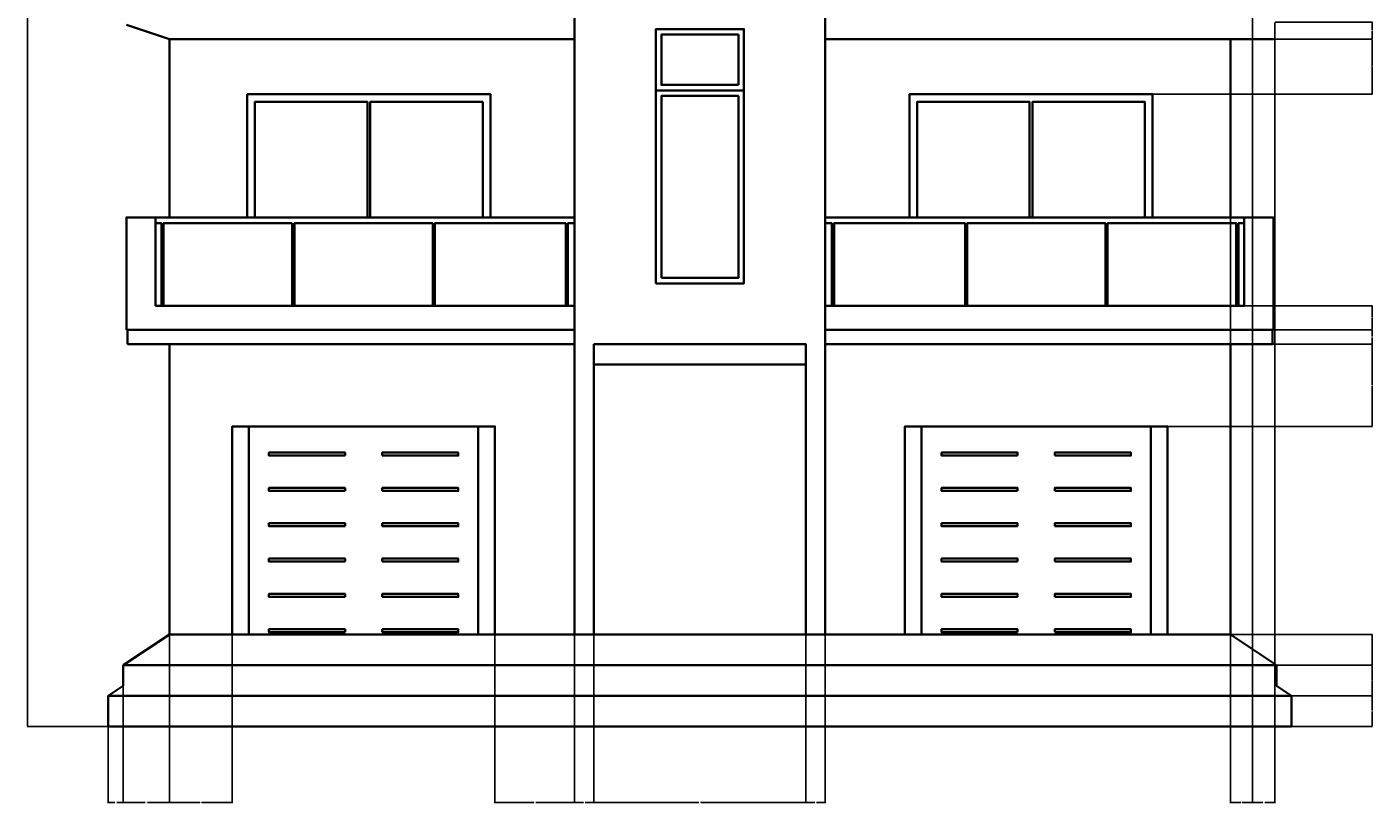
# Model space of a CAD drawing. Units: feet. Extents: x 2893 to 4112, y 897 to 1573.
# Tile 6 of 7: x 3556 to 4112, y 897 to 1218. Entities that reach past the tile are written whole.
import ezdxf

# ---------------------------------------------------------------- set-up
doc = ezdxf.new("R2010")
doc.units = ezdxf.units.FT
doc.layers.add('A-ANNO-DIMS', color=2, linetype='Continuous', lineweight=18)
doc.layers.add('A-ELEV', color=7, linetype='Continuous', lineweight=35)
doc.styles.get("Standard").update_dxf_attribs({"font": 'arial.ttf'})
doc.dimstyles.get("Standard").update_dxf_attribs({"dimtxt": 0.18, "dimasz": 0.18, "dimexe": 0.18, "dimexo": 0.0625, "dimgap": 0.09, "dimtad": 0, "dimtih": 1, "dimtoh": 1, "dimdec": 1, "dimzin": 0, "dimdsep": 46, "dimlunit": 3, "dimtxsty": 'Standard', "dimcen": 0.09, "dimadec": 0, "dimazin": 0, "dimtfac": 1, "dimtdec": 1, "dimtofl": 0, "dimtmove": 0, "dimatfit": 3, "dimfxl": 1, "dimtolj": 1, "dimtzin": 0, "dimarcsym": 0})

# ---------------------------------------------------------------- blocks, each defined once
blk = doc.blocks.new('*D14')
at = {"layer": 'A-ANNO-DIMS', "color": 0, "lineweight": -2, "transparency": 16777216}
for p, q in [((3587.66, 1527.89), (3556.04, 1527.89)), ((3556.22, 1527.71), (3556.22, 1228.65)), ((3556.22, 929.23), (3556.22, 1228.29)), ((3589.45, 929.05), (3556.04, 929.05))]:
    blk.add_line(p, q, dxfattribs=at)
at = {"layer": 'A-ANNO-DIMS', "color": 0, "transparency": 16777216}
for points in [[(3556.19, 1527.71), (3556.25, 1527.71), (3556.22, 1527.89)], [(3556.19, 929.23), (3556.25, 929.23), (3556.22, 929.05)]]:
    blk.add_solid(points, dxfattribs=at)
at = {"layer": 'Defpoints', "color": 0, "transparency": 16777216}
for p in [(3556.22, 1527.89), (3587.72, 1527.89), (3589.51, 929.05)]:
    blk.add_point(p, dxfattribs=at)
at = {"layer": 'A-ANNO-DIMS', "color": 0, "transparency": 16777216, "insert": (3556.22, 1228.47), "char_height": 0.18, "attachment_point": 5}
blk.add_mtext('\\A1;598.8', dxfattribs=at)
blk = doc.blocks.new('*D16')
at = {"layer": 'A-ANNO-DIMS', "color": 0, "lineweight": -2, "transparency": 16777216}
for p, q in [((3595.77, 954.3), (3595.77, 897.37)), ((3589.51, 941.64), (3589.51, 897.37)), ((3589.69, 897.55), (3592.25, 897.55)), ((3595.59, 897.55), (3593.03, 897.55))]:
    blk.add_line(p, q, dxfattribs=at)
at = {"layer": 'A-ANNO-DIMS', "color": 0, "transparency": 16777216}
for points in [[(3589.69, 897.58), (3589.69, 897.52), (3589.51, 897.55)], [(3595.59, 897.58), (3595.59, 897.52), (3595.77, 897.55)]]:
    blk.add_solid(points, dxfattribs=at)
at = {"layer": 'Defpoints', "color": 0, "transparency": 16777216}
for p in [(3595.77, 954.36), (3589.51, 941.7), (3595.77, 897.55)]:
    blk.add_point(p, dxfattribs=at)
at = {"layer": 'A-ANNO-DIMS', "color": 0, "transparency": 16777216, "insert": (3592.64, 897.55), "char_height": 0.18, "attachment_point": 5}
blk.add_mtext('\\A1;6.263', dxfattribs=at)
blk = doc.blocks.new('*D17')
at = {"layer": 'A-ANNO-DIMS', "color": 0, "lineweight": -2, "transparency": 16777216}
for p, q in [((3614.84, 966.95), (3614.84, 897.37)), ((3595.77, 954.3), (3595.77, 897.37)), ((3595.95, 897.55), (3604.85, 897.55)), ((3614.66, 897.55), (3605.76, 897.55))]:
    blk.add_line(p, q, dxfattribs=at)
at = {"layer": 'A-ANNO-DIMS', "color": 0, "transparency": 16777216}
for points in [[(3595.95, 897.58), (3595.95, 897.52), (3595.77, 897.55)], [(3614.66, 897.58), (3614.66, 897.52), (3614.84, 897.55)]]:
    blk.add_solid(points, dxfattribs=at)
at = {"layer": 'Defpoints', "color": 0, "transparency": 16777216}
for p in [(3614.84, 967.01), (3595.77, 954.36), (3614.84, 897.55)]:
    blk.add_point(p, dxfattribs=at)
at = {"layer": 'A-ANNO-DIMS', "color": 0, "transparency": 16777216, "insert": (3605.3, 897.55), "char_height": 0.18, "attachment_point": 5}
blk.add_mtext('\\A1;19.063', dxfattribs=at)
blk = doc.blocks.new('*D18')
at = {"layer": 'A-ANNO-DIMS', "color": 0, "lineweight": -2, "transparency": 16777216}
for p, q in [((3614.84, 966.95), (3614.84, 897.37)), ((3640.81, 966.95), (3640.81, 897.37)), ((3615.02, 897.55), (3627.43, 897.55)), ((3640.63, 897.55), (3628.22, 897.55))]:
    blk.add_line(p, q, dxfattribs=at)
at = {"layer": 'A-ANNO-DIMS', "color": 0, "transparency": 16777216}
for points in [[(3615.02, 897.58), (3615.02, 897.52), (3614.84, 897.55)], [(3640.63, 897.58), (3640.63, 897.52), (3640.81, 897.55)]]:
    blk.add_solid(points, dxfattribs=at)
at = {"layer": 'Defpoints', "color": 0, "transparency": 16777216}
for p in [(3614.84, 967.01), (3640.81, 967.01), (3640.81, 897.55)]:
    blk.add_point(p, dxfattribs=at)
at = {"layer": 'A-ANNO-DIMS', "color": 0, "transparency": 16777216, "insert": (3627.82, 897.55), "char_height": 0.18, "attachment_point": 5}
blk.add_mtext('\\A1;25.98', dxfattribs=at)
blk = doc.blocks.new('*D19')
at = {"layer": 'A-ANNO-DIMS', "color": 0, "lineweight": -2, "transparency": 16777216}
for p, q in [((3749.39, 966.95), (3749.39, 897.37)), ((3782.33, 966.95), (3782.33, 897.37)), ((3749.57, 897.55), (3765.47, 897.55)), ((3782.15, 897.55), (3766.25, 897.55))]:
    blk.add_line(p, q, dxfattribs=at)
at = {"layer": 'A-ANNO-DIMS', "color": 0, "transparency": 16777216}
for points in [[(3749.57, 897.58), (3749.57, 897.52), (3749.39, 897.55)], [(3782.15, 897.58), (3782.15, 897.52), (3782.33, 897.55)]]:
    blk.add_solid(points, dxfattribs=at)
at = {"layer": 'Defpoints', "color": 0, "transparency": 16777216}
for p in [(3749.39, 967.01), (3782.33, 967.01), (3782.33, 897.55)]:
    blk.add_point(p, dxfattribs=at)
at = {"layer": 'A-ANNO-DIMS', "color": 0, "transparency": 16777216, "insert": (3765.86, 897.55), "char_height": 0.18, "attachment_point": 5}
blk.add_mtext('\\A1;32.94', dxfattribs=at)
blk = doc.blocks.new('*D20')
at = {"layer": 'A-ANNO-DIMS', "color": 0, "lineweight": -2, "transparency": 16777216}
for p, q in [((3782.33, 966.95), (3782.33, 897.37)), ((3790.32, 966.95), (3790.32, 897.37)), ((3782.51, 897.55), (3786, 897.55)), ((3790.14, 897.55), (3786.65, 897.55))]:
    blk.add_line(p, q, dxfattribs=at)
at = {"layer": 'A-ANNO-DIMS', "color": 0, "transparency": 16777216}
for points in [[(3782.51, 897.58), (3782.51, 897.52), (3782.33, 897.55)], [(3790.14, 897.58), (3790.14, 897.52), (3790.32, 897.55)]]:
    blk.add_solid(points, dxfattribs=at)
at = {"layer": 'Defpoints', "color": 0, "transparency": 16777216}
for p in [(3782.33, 967.01), (3790.32, 967.01), (3790.32, 897.55)]:
    blk.add_point(p, dxfattribs=at)
at = {"layer": 'A-ANNO-DIMS', "color": 0, "transparency": 16777216, "insert": (3786.32, 897.55), "char_height": 0.18, "attachment_point": 5}
blk.add_mtext('\\A1;7.99', dxfattribs=at)
blk = doc.blocks.new('*D21')
at = {"layer": 'A-ANNO-DIMS', "color": 0, "lineweight": -2, "transparency": 16777216}
for p, q in [((3790.32, 966.95), (3790.32, 897.37)), ((3877.97, 966.95), (3877.97, 897.37)), ((3790.5, 897.55), (3833.75, 897.55)), ((3877.79, 897.55), (3834.54, 897.55))]:
    blk.add_line(p, q, dxfattribs=at)
at = {"layer": 'A-ANNO-DIMS', "color": 0, "transparency": 16777216}
for points in [[(3790.5, 897.58), (3790.5, 897.52), (3790.32, 897.55)], [(3877.79, 897.58), (3877.79, 897.52), (3877.97, 897.55)]]:
    blk.add_solid(points, dxfattribs=at)
at = {"layer": 'Defpoints', "color": 0, "transparency": 16777216}
for p in [(3790.32, 967.01), (3877.97, 967.01), (3877.97, 897.55)]:
    blk.add_point(p, dxfattribs=at)
at = {"layer": 'A-ANNO-DIMS', "color": 0, "transparency": 16777216, "insert": (3834.14, 897.55), "char_height": 0.18, "attachment_point": 5}
blk.add_mtext('\\A1;87.65', dxfattribs=at)
blk = doc.blocks.new('*D22')
at = {"layer": 'A-ANNO-DIMS', "color": 0, "lineweight": -2, "transparency": 16777216}
for p, q in [((3877.97, 966.95), (3877.97, 897.37)), ((3885.96, 966.95), (3885.96, 897.37)), ((3878.15, 897.55), (3881.64, 897.55)), ((3885.78, 897.55), (3882.29, 897.55))]:
    blk.add_line(p, q, dxfattribs=at)
at = {"layer": 'A-ANNO-DIMS', "color": 0, "transparency": 16777216}
for points in [[(3878.15, 897.58), (3878.15, 897.52), (3877.97, 897.55)], [(3885.78, 897.58), (3885.78, 897.52), (3885.96, 897.55)]]:
    blk.add_solid(points, dxfattribs=at)
at = {"layer": 'Defpoints', "color": 0, "transparency": 16777216}
for p in [(3877.97, 967.01), (3885.96, 967.01), (3885.96, 897.55)]:
    blk.add_point(p, dxfattribs=at)
at = {"layer": 'A-ANNO-DIMS', "color": 0, "transparency": 16777216, "insert": (3881.97, 897.55), "char_height": 0.18, "attachment_point": 5}
blk.add_mtext('\\A1;7.99', dxfattribs=at)
blk = doc.blocks.new('*D23')
at = {"layer": 'A-ANNO-DIMS', "color": 0, "lineweight": -2, "transparency": 16777216}
for p, q in [((4062.6, 1232.06), (4062.6, 897.37)), ((4053.45, 1212.95), (4053.45, 897.37)), ((4053.63, 897.55), (4057.7, 897.55)), ((4062.42, 897.55), (4058.35, 897.55))]:
    blk.add_line(p, q, dxfattribs=at)
at = {"layer": 'A-ANNO-DIMS', "color": 0, "transparency": 16777216}
for points in [[(4053.63, 897.58), (4053.63, 897.52), (4053.45, 897.55)], [(4062.42, 897.58), (4062.42, 897.52), (4062.6, 897.55)]]:
    blk.add_solid(points, dxfattribs=at)
at = {"layer": 'Defpoints', "color": 0, "transparency": 16777216}
for p in [(4062.6, 1232.12), (4053.45, 1213.01), (4062.6, 897.55)]:
    blk.add_point(p, dxfattribs=at)
at = {"layer": 'A-ANNO-DIMS', "color": 0, "transparency": 16777216, "insert": (4058.03, 897.55), "char_height": 0.18, "attachment_point": 5}
blk.add_mtext('\\A1;9.15', dxfattribs=at)
blk = doc.blocks.new('*D24')
at = {"layer": 'A-ANNO-DIMS', "color": 0, "lineweight": -2, "transparency": 16777216}
for p, q in [((4062.6, 1232.06), (4062.6, 897.37)), ((4071.89, 1220.03), (4071.89, 897.37)), ((4062.78, 897.55), (4066.85, 897.55)), ((4071.71, 897.55), (4067.64, 897.55))]:
    blk.add_line(p, q, dxfattribs=at)
at = {"layer": 'A-ANNO-DIMS', "color": 0, "transparency": 16777216}
for points in [[(4062.78, 897.58), (4062.78, 897.52), (4062.6, 897.55)], [(4071.71, 897.58), (4071.71, 897.52), (4071.89, 897.55)]]:
    blk.add_solid(points, dxfattribs=at)
at = {"layer": 'Defpoints', "color": 0, "transparency": 16777216}
for p in [(4062.6, 1232.12), (4071.89, 1220.09), (4071.89, 897.55)]:
    blk.add_point(p, dxfattribs=at)
at = {"layer": 'A-ANNO-DIMS', "color": 0, "transparency": 16777216, "insert": (4067.25, 897.55), "char_height": 0.18, "attachment_point": 5}
blk.add_mtext('\\A1;9.288', dxfattribs=at)
blk = doc.blocks.new('*D25')
at = {"layer": 'A-ANNO-DIMS', "color": 0, "lineweight": -2, "transparency": 16777216}
for p, q in [((4078.84, 941.7), (4112.25, 941.7)), ((4112.07, 941.52), (4112.07, 935.56)), ((4112.07, 929.23), (4112.07, 935.2)), ((4078.84, 929.05), (4112.25, 929.05))]:
    blk.add_line(p, q, dxfattribs=at)
at = {"layer": 'A-ANNO-DIMS', "color": 0, "transparency": 16777216}
for points in [[(4112.04, 941.52), (4112.1, 941.52), (4112.07, 941.7)], [(4112.04, 929.23), (4112.1, 929.23), (4112.07, 929.05)]]:
    blk.add_solid(points, dxfattribs=at)
at = {"layer": 'Defpoints', "color": 0, "transparency": 16777216}
for p in [(4078.78, 941.7), (4112.07, 941.7), (4078.78, 929.05)]:
    blk.add_point(p, dxfattribs=at)
at = {"layer": 'A-ANNO-DIMS', "color": 0, "transparency": 16777216, "insert": (4112.07, 935.38), "char_height": 0.18, "attachment_point": 5}
blk.add_mtext('\\A1;12.655', dxfattribs=at)
blk = doc.blocks.new('*D26')
at = {"layer": 'A-ANNO-DIMS', "color": 0, "lineweight": -2, "transparency": 16777216}
for p, q in [((4072.58, 954.36), (4112.25, 954.36)), ((4112.07, 954.18), (4112.07, 948.21)), ((4112.07, 941.88), (4112.07, 947.85)), ((4078.84, 941.7), (4112.25, 941.7))]:
    blk.add_line(p, q, dxfattribs=at)
at = {"layer": 'A-ANNO-DIMS', "color": 0, "transparency": 16777216}
for points in [[(4112.04, 954.18), (4112.1, 954.18), (4112.07, 954.36)], [(4112.04, 941.88), (4112.1, 941.88), (4112.07, 941.7)]]:
    blk.add_solid(points, dxfattribs=at)
at = {"layer": 'Defpoints', "color": 0, "transparency": 16777216}
for p in [(4072.52, 954.36), (4112.07, 954.36), (4078.78, 941.7)]:
    blk.add_point(p, dxfattribs=at)
at = {"layer": 'A-ANNO-DIMS', "color": 0, "transparency": 16777216, "insert": (4112.07, 948.03), "char_height": 0.18, "attachment_point": 5}
blk.add_mtext('\\A1;12.655', dxfattribs=at)
blk = doc.blocks.new('*D27')
at = {"layer": 'A-ANNO-DIMS', "color": 0, "lineweight": -2, "transparency": 16777216}
for p, q in [((4053.52, 967.01), (4112.25, 967.01)), ((4112.07, 966.83), (4112.07, 960.87)), ((4112.07, 954.54), (4112.07, 960.51)), ((4072.58, 954.36), (4112.25, 954.36))]:
    blk.add_line(p, q, dxfattribs=at)
at = {"layer": 'A-ANNO-DIMS', "color": 0, "transparency": 16777216}
for points in [[(4112.04, 966.83), (4112.1, 966.83), (4112.07, 967.01)], [(4112.04, 954.54), (4112.1, 954.54), (4112.07, 954.36)]]:
    blk.add_solid(points, dxfattribs=at)
at = {"layer": 'Defpoints', "color": 0, "transparency": 16777216}
for p in [(4053.45, 967.01), (4112.07, 967.01), (4072.52, 954.36)]:
    blk.add_point(p, dxfattribs=at)
at = {"layer": 'A-ANNO-DIMS', "color": 0, "transparency": 16777216, "insert": (4112.07, 960.69), "char_height": 0.18, "attachment_point": 5}
blk.add_mtext('\\A1;12.655', dxfattribs=at)
blk = doc.blocks.new('*D28')
at = {"layer": 'A-ANNO-DIMS', "color": 0, "lineweight": -2, "transparency": 16777216}
for p, q in [((4070.88, 1087.01), (4112.25, 1087.01)), ((4112.07, 1086.83), (4112.07, 1070.21)), ((4112.07, 1053.22), (4112.07, 1069.84)), ((4027.54, 1053.04), (4112.25, 1053.04))]:
    blk.add_line(p, q, dxfattribs=at)
at = {"layer": 'A-ANNO-DIMS', "color": 0, "transparency": 16777216}
for points in [[(4112.04, 1086.83), (4112.1, 1086.83), (4112.07, 1087.01)], [(4112.04, 1053.22), (4112.1, 1053.22), (4112.07, 1053.04)]]:
    blk.add_solid(points, dxfattribs=at)
at = {"layer": 'Defpoints', "color": 0, "transparency": 16777216}
for p in [(4070.82, 1087.01), (4112.07, 1087.01), (4027.48, 1053.04)]:
    blk.add_point(p, dxfattribs=at)
at = {"layer": 'A-ANNO-DIMS', "color": 0, "transparency": 16777216, "insert": (4112.07, 1070.03), "char_height": 0.18, "attachment_point": 5}
blk.add_mtext('\\A1;33.98', dxfattribs=at)
blk = doc.blocks.new('*D29')
at = {"layer": 'A-ANNO-DIMS', "color": 0, "lineweight": -2, "transparency": 16777216}
for p, q in [((4070.88, 1093.01), (4112.25, 1093.01)), ((4112.07, 1092.83), (4112.07, 1090.2)), ((4070.88, 1087.01), (4112.25, 1087.01)), ((4112.07, 1087.19), (4112.07, 1089.83))]:
    blk.add_line(p, q, dxfattribs=at)
at = {"layer": 'A-ANNO-DIMS', "color": 0, "transparency": 16777216}
for points in [[(4112.04, 1092.83), (4112.1, 1092.83), (4112.07, 1093.01)], [(4112.04, 1087.19), (4112.1, 1087.19), (4112.07, 1087.01)]]:
    blk.add_solid(points, dxfattribs=at)
at = {"layer": 'Defpoints', "color": 0, "transparency": 16777216}
for p in [(4070.82, 1093.01), (4112.07, 1093.01), (4070.82, 1087.01)]:
    blk.add_point(p, dxfattribs=at)
at = {"layer": 'A-ANNO-DIMS', "color": 0, "transparency": 16777216, "insert": (4112.07, 1090.01), "char_height": 0.18, "attachment_point": 5}
blk.add_mtext('\\A1;6', dxfattribs=at)
blk = doc.blocks.new('*D30')
at = {"layer": 'A-ANNO-DIMS', "color": 0, "lineweight": -2, "transparency": 16777216}
for p, q in [((4059.27, 1102.93), (4112.25, 1102.93)), ((4112.07, 1102.75), (4112.07, 1098.15)), ((4112.07, 1093.19), (4112.07, 1097.79)), ((4070.88, 1093.01), (4112.25, 1093.01))]:
    blk.add_line(p, q, dxfattribs=at)
at = {"layer": 'A-ANNO-DIMS', "color": 0, "transparency": 16777216}
for points in [[(4112.04, 1102.75), (4112.1, 1102.75), (4112.07, 1102.93)], [(4112.04, 1093.19), (4112.1, 1093.19), (4112.07, 1093.01)]]:
    blk.add_solid(points, dxfattribs=at)
at = {"layer": 'Defpoints', "color": 0, "transparency": 16777216}
for p in [(4059.21, 1102.93), (4112.07, 1102.93), (4070.82, 1093.01)]:
    blk.add_point(p, dxfattribs=at)
at = {"layer": 'A-ANNO-DIMS', "color": 0, "transparency": 16777216, "insert": (4112.07, 1097.97), "char_height": 0.18, "attachment_point": 5}
blk.add_mtext('\\A1;9.916', dxfattribs=at)
blk = doc.blocks.new('*D31')
at = {"layer": 'A-ANNO-DIMS', "color": 0, "lineweight": -2, "transparency": 16777216}
for p, q in [((4071.32, 1213.01), (4112.25, 1213.01)), ((4112.07, 1212.83), (4112.07, 1201.83)), ((4112.07, 1190.47), (4112.07, 1201.47)), ((4021.33, 1190.29), (4112.25, 1190.29))]:
    blk.add_line(p, q, dxfattribs=at)
at = {"layer": 'A-ANNO-DIMS', "color": 0, "transparency": 16777216}
for points in [[(4112.04, 1212.83), (4112.1, 1212.83), (4112.07, 1213.01)], [(4112.04, 1190.47), (4112.1, 1190.47), (4112.07, 1190.29)]]:
    blk.add_solid(points, dxfattribs=at)
at = {"layer": 'Defpoints', "color": 0, "transparency": 16777216}
for p in [(4071.26, 1213.01), (4112.07, 1213.01), (4021.27, 1190.29)]:
    blk.add_point(p, dxfattribs=at)
at = {"layer": 'A-ANNO-DIMS', "color": 0, "transparency": 16777216, "insert": (4112.07, 1201.65), "char_height": 0.18, "attachment_point": 5}
blk.add_mtext('\\A1;22.722', dxfattribs=at)
blk = doc.blocks.new('*D32')
at = {"layer": 'A-ANNO-DIMS', "color": 0, "lineweight": -2, "transparency": 16777216}
for p, q in [((4071.95, 1220.09), (4112.25, 1220.09)), ((4112.07, 1219.91), (4112.07, 1216.74)), ((4112.07, 1213.19), (4112.07, 1216.37)), ((4071.32, 1213.01), (4112.25, 1213.01))]:
    blk.add_line(p, q, dxfattribs=at)
at = {"layer": 'A-ANNO-DIMS', "color": 0, "transparency": 16777216}
for points in [[(4112.04, 1219.91), (4112.1, 1219.91), (4112.07, 1220.09)], [(4112.04, 1213.19), (4112.1, 1213.19), (4112.07, 1213.01)]]:
    blk.add_solid(points, dxfattribs=at)
at = {"layer": 'Defpoints', "color": 0, "transparency": 16777216}
for p in [(4071.89, 1220.09), (4112.07, 1220.09), (4071.26, 1213.01)]:
    blk.add_point(p, dxfattribs=at)
at = {"layer": 'A-ANNO-DIMS', "color": 0, "transparency": 16777216, "insert": (4112.07, 1216.55), "char_height": 0.18, "attachment_point": 5}
blk.add_mtext('\\A1;7.08', dxfattribs=at)

msp = doc.modelspace()

# ---------------------------------------------------------------- linework, layer by layer
at = {"layer": 'A-ELEV'}
for p, q in [((3782.3275, 967.0143), (3782.3275, 1541.1646)), ((3885.9608, 967.0143), (3885.9608, 1541.1646)), ((3614.8353, 1213.0143), (3597.0307, 1219.0143)), ((3614.8353, 1213.0143), (3782.3275, 1213.0143)), ((3614.8353, 1139.3799), (3614.8353, 1213.0143)), ((3614.8353, 1213.0143), (3614.8353, 1139.3799)), ((3885.9608, 1213.0143), (4071.2577, 1213.0143)), ((4053.4531, 1213.0143), (4053.4531, 1139.3799)), ((3597.0307, 1093.0143), (3597.0307, 1139.3799)), ((3782.3275, 1093.0143), (3597.0307, 1093.0143)), ((3885.9608, 1093.0143), (4071.2577, 1093.0143)), ((3782.3275, 1087.0143), (3597.4699, 1087.0143)), ((3877.9713, 1087.0143), (3790.317, 1087.0143)), ((4070.8185, 1087.0143), (3885.9608, 1087.0143)), ((3595.7722, 954.3595), (3614.8353, 967.0143)), ((3614.8353, 967.0143), (4053.4531, 967.0143)), ((4072.5162, 954.3595), (4053.4531, 967.0143)), ((3589.5092, 941.7047), (3595.7722, 945.8624)), ((3589.5092, 941.7047), (3589.5092, 929.0499)), ((4078.7792, 941.7047), (4072.5162, 945.8624)), ((4078.7792, 941.7047), (4078.7792, 929.0499))]:
    msp.add_line(p, q, dxfattribs=at)
for points in [[(3852.3189, 1191.9186), (3815.9695, 1191.9186), (3815.9695, 1217.2478), (3852.3189, 1217.2478)], [(3850.0494, 1194.1881), (3818.239, 1194.1881), (3818.239, 1214.9783), (3850.0494, 1214.9783)], [(3815.9695, 1112.1098), (3852.3189, 1112.1098), (3852.3189, 1191.9186), (3815.9695, 1191.9186)], [(3747.5019, 1139.3799), (3647.022, 1139.3799), (3647.022, 1190.2919), (3747.5019, 1190.2919)], [(3818.239, 1114.3793), (3850.0494, 1114.3793), (3850.0494, 1189.6491), (3818.239, 1189.6491)], [(3920.7865, 1139.3799), (4021.2664, 1139.3799), (4021.2664, 1190.2919), (3920.7865, 1190.2919)], [(3665.6357, 1136.9984), (3612.3836, 1136.9984), (3612.3836, 1102.9302), (3611.5098, 1102.9302), (3611.5098, 1136.9984), (3609.0791, 1136.9984), (3609.0791, 1139.3799), (3782.3275, 1139.3799), (3782.3275, 1136.9984), (3779.5608, 1136.9984), (3779.5608, 1102.9302), (3778.687, 1102.9302), (3778.687, 1136.9984), (3724.5465, 1136.9984), (3724.5465, 1102.9302), (3723.6728, 1102.9302), (3723.6728, 1136.9984), (3666.5095, 1136.9984), (3666.5095, 1102.9302), (3665.6357, 1102.9302)], [(4002.6527, 1136.9984), (4055.9048, 1136.9984), (4055.9048, 1102.9302), (4056.7785, 1102.9302), (4056.7785, 1136.9984), (4059.2093, 1136.9984), (4059.2093, 1139.3799), (3885.9608, 1139.3799), (3885.9608, 1136.9984), (3888.7276, 1136.9984), (3888.7276, 1102.9302), (3889.6014, 1102.9302), (3889.6014, 1136.9984), (3943.7418, 1136.9984), (3943.7418, 1102.9302), (3944.6156, 1102.9302), (3944.6156, 1136.9984), (4001.7789, 1136.9984), (4001.7789, 1102.9302), (4002.6527, 1102.9302)], [(3790.317, 1087.0143), (3877.9713, 1087.0143), (3877.9713, 967.0143), (3790.317, 967.0143)], [(3790.317, 1087.0143), (3877.9713, 1087.0143), (3877.9713, 1078.6766), (3790.317, 1078.6766)], [(4053.4531, 967.0143), (3885.9608, 967.0143), (3885.9608, 1087.0143), (4053.4531, 1087.0143)], [(3749.3905, 967.0143), (3640.8129, 967.0143), (3640.8129, 1053.0375), (3749.3905, 1053.0375)], [(3640.8129, 1053.0375), (3647.6811, 1053.0375), (3647.6811, 967.0143), (3640.8129, 967.0143)], [(3749.3905, 1053.0375), (3742.5223, 1053.0375), (3742.5223, 967.0143), (3749.3905, 967.0143)], [(3918.8979, 967.0143), (4027.4755, 967.0143), (4027.4755, 1053.0375), (3918.8979, 1053.0375)], [(3918.8979, 1053.0375), (3925.7661, 1053.0375), (3925.7661, 967.0143), (3918.8979, 967.0143)], [(4027.4755, 1053.0375), (4020.6073, 1053.0375), (4020.6073, 967.0143), (4027.4755, 967.0143)], [(3687.4156, 1040.9943), (3655.944, 1040.9943), (3655.944, 1042.2356), (3687.4156, 1042.2356)], [(3702.7878, 1040.9943), (3734.2594, 1040.9943), (3734.2594, 1042.2356), (3702.7878, 1042.2356)], [(3965.5006, 1040.9943), (3934.029, 1040.9943), (3934.029, 1042.2356), (3965.5006, 1042.2356)], [(3980.8728, 1040.9943), (4012.3444, 1040.9943), (4012.3444, 1042.2356), (3980.8728, 1042.2356)], [(3687.4156, 1026.3833), (3655.944, 1026.3833), (3655.944, 1027.6246), (3687.4156, 1027.6246)], [(3702.7878, 1026.3833), (3734.2594, 1026.3833), (3734.2594, 1027.6246), (3702.7878, 1027.6246)], [(3965.5006, 1026.3833), (3934.029, 1026.3833), (3934.029, 1027.6246), (3965.5006, 1027.6246)], [(3980.8728, 1026.3833), (4012.3444, 1026.3833), (4012.3444, 1027.6246), (3980.8728, 1027.6246)], [(3687.4156, 1011.7724), (3655.944, 1011.7724), (3655.944, 1013.0137), (3687.4156, 1013.0137)], [(3702.7878, 1011.7724), (3734.2594, 1011.7724), (3734.2594, 1013.0137), (3702.7878, 1013.0137)], [(3965.5006, 1011.7724), (3934.029, 1011.7724), (3934.029, 1013.0137), (3965.5006, 1013.0137)], [(3980.8728, 1011.7724), (4012.3444, 1011.7724), (4012.3444, 1013.0137), (3980.8728, 1013.0137)], [(3687.4156, 997.1615), (3655.944, 997.1615), (3655.944, 998.4028), (3687.4156, 998.4028)], [(3702.7878, 997.1615), (3734.2594, 997.1615), (3734.2594, 998.4028), (3702.7878, 998.4028)], [(3965.5006, 997.1615), (3934.029, 997.1615), (3934.029, 998.4028), (3965.5006, 998.4028)], [(3980.8728, 997.1615), (4012.3444, 997.1615), (4012.3444, 998.4028), (3980.8728, 998.4028)], [(3687.4156, 982.5506), (3655.944, 982.5506), (3655.944, 983.7919), (3687.4156, 983.7919)], [(3702.7878, 982.5506), (3734.2594, 982.5506), (3734.2594, 983.7919), (3702.7878, 983.7919)], [(3965.5006, 982.5506), (3934.029, 982.5506), (3934.029, 983.7919), (3965.5006, 983.7919)], [(3980.8728, 982.5506), (4012.3444, 982.5506), (4012.3444, 983.7919), (3980.8728, 983.7919)], [(3687.4156, 967.9397), (3655.944, 967.9397), (3655.944, 969.181), (3687.4156, 969.181)], [(3702.7878, 967.9397), (3734.2594, 967.9397), (3734.2594, 969.181), (3702.7878, 969.181)], [(3965.5006, 967.9397), (3934.029, 967.9397), (3934.029, 969.181), (3965.5006, 969.181)], [(3980.8728, 967.9397), (4012.3444, 967.9397), (4012.3444, 969.181), (3980.8728, 969.181)]]:
    msp.add_lwpolyline(points, close=True, dxfattribs=at)
for points in [[(3744.3518, 1139.3799), (3744.3518, 1187.1419), (3697.8342, 1187.1419), (3697.8342, 1139.3799), (3696.6897, 1139.3799), (3696.6897, 1187.1419), (3650.1721, 1187.1419), (3650.1721, 1139.3799)], [(3923.9365, 1139.3799), (3923.9365, 1187.1419), (3970.4542, 1187.1419), (3970.4542, 1139.3799), (3971.5986, 1139.3799), (3971.5986, 1187.1419), (4018.1163, 1187.1419), (4018.1163, 1139.3799)], [(3609.0791, 1102.9302), (3609.0791, 1139.3799), (3597.0307, 1139.3799), (3597.0307, 1093.0143)], [(4059.2093, 1102.9302), (4059.2093, 1139.3799), (4071.2577, 1139.3799), (4071.2577, 1093.0143)], [(3597.0307, 1102.9302), (3597.0307, 1093.0143)], [(3782.3275, 1087.0143), (3782.3275, 1102.9302), (3609.0791, 1102.9302)], [(3885.9608, 1087.0143), (3885.9608, 1102.9302), (4059.2093, 1102.9302)], [(3597.4699, 1087.0143), (3597.4699, 1093.0143)], [(3782.3275, 1093.0143), (3782.3275, 1087.0143)], [(4070.8185, 1087.0143), (4070.8185, 1093.0143)], [(3614.8353, 1087.0143), (3614.8353, 967.0143), (3782.3275, 967.0143), (3782.3275, 1087.0143)], [(3696.8415, 967.0143), (3693.3618, 967.0143)], [(3595.7722, 945.8624), (3595.7722, 954.3595), (4072.5162, 954.3595), (4072.5162, 945.8624)], [(3589.5092, 941.7047), (4078.7792, 941.7047)], [(4072.5162, 941.7047), (3595.7722, 941.7047)], [(4078.7792, 929.0499), (3589.5092, 929.0499)]]:
    msp.add_lwpolyline(points, dxfattribs=at)

# ---------------------------------------------------------------- dimensions: what is measured, and where the dimension line sits
at = {"layer": 'A-ANNO-DIMS'}
for base, p1, p2, override, picture, middle in [((3556.2226, 1527.889), (3589.5092, 929.0499), (3587.7226, 1527.889), {"dimdec": 1, "dimlfac": 1, "dimrnd": 0, "dimzin": 0, "dimdsep": 46, "dimlunit": 2}, '*D14', (3556.2226, 1228.4695)), ((4112.0657, 1220.0947), (4071.2577, 1213.0143), (4071.8918, 1220.0947), {"dimdec": 2, "dimlfac": 1, "dimrnd": 0, "dimzin": 0, "dimdsep": 46, "dimlunit": 2}, '*D32', (4112.0657, 1216.5545)), ((4112.0657, 1213.0143), (4021.2664, 1190.2919), (4071.2577, 1213.0143), {"dimdec": 3, "dimlfac": 1, "dimrnd": 0, "dimzin": 0, "dimdsep": 46, "dimlunit": 2}, '*D31', (4112.0657, 1201.6531)), ((4112.0657, 1102.9302), (4070.8185, 1093.0143), (4059.2093, 1102.9302), {"dimdec": 3, "dimlfac": 1, "dimrnd": 0, "dimzin": 0, "dimdsep": 46, "dimlunit": 2}, '*D30', (4112.0657, 1097.9723)), ((4112.0657, 1093.0143), (4070.8185, 1087.0143), (4070.8185, 1093.0143), {"dimdec": 0, "dimlfac": 1, "dimrnd": 0, "dimzin": 0, "dimdsep": 46, "dimlunit": 2}, '*D29', (4112.0657, 1090.0143)), ((4112.0657, 1087.0143), (4027.4755, 1053.0375), (4070.8185, 1087.0143), {"dimdec": 2, "dimlfac": 1, "dimrnd": 0, "dimzin": 0, "dimdsep": 46, "dimlunit": 2}, '*D28', (4112.0657, 1070.0259)), ((4112.0657, 967.0143), (4072.5162, 954.3595), (4053.4531, 967.0143), {"dimdec": 3, "dimlfac": 1, "dimrnd": 0, "dimzin": 0, "dimdsep": 46, "dimlunit": 2}, '*D27', (4112.0657, 960.6869)), ((4112.0657, 954.3595), (4078.7792, 941.7047), (4072.5162, 954.3595), {"dimdec": 3, "dimlfac": 1, "dimrnd": 0, "dimzin": 0, "dimdsep": 46, "dimlunit": 2}, '*D26', (4112.0657, 948.0321)), ((4112.0657, 941.7047), (4078.7792, 929.0499), (4078.7792, 941.7047), {"dimdec": 3, "dimlfac": 1, "dimrnd": 0, "dimzin": 0, "dimdsep": 46, "dimlunit": 2}, '*D25', (4112.0657, 935.3773))]:
    dim = msp.add_linear_dim(base=base, p1=p1, p2=p2, angle=90, dimstyle='Standard', override=override, dxfattribs=at)
    dim.commit()
    dim.dimension.update_dxf_attribs({"geometry": picture, "text_midpoint": middle})
for base, p1, p2, override, picture, middle in [((4062.6038, 897.5499), (4053.4531, 1213.0143), (4062.6038, 1232.1197), {"dimdec": 2, "dimlfac": 1, "dimrnd": 0, "dimzin": 0, "dimdsep": 46, "dimlunit": 2}, '*D23', (4058.0285, 897.5499)), ((4071.8918, 897.5499), (4062.6038, 1232.1197), (4071.8918, 1220.0947), {"dimdec": 3, "dimlfac": 1, "dimrnd": 0, "dimzin": 0, "dimdsep": 46, "dimlunit": 2}, '*D24', (4067.2478, 897.5499)), ((3614.8353, 897.5499), (3595.7722, 954.3595), (3614.8353, 967.0143), {"dimdec": 3, "dimlfac": 1, "dimrnd": 0, "dimzin": 0, "dimdsep": 46, "dimlunit": 2}, '*D17', (3605.3037, 897.5499)), ((3640.8129, 897.5499), (3614.8353, 967.0143), (3640.8129, 967.0143), {"dimdec": 2, "dimlfac": 1, "dimrnd": 0, "dimzin": 0, "dimdsep": 46, "dimlunit": 2}, '*D18', (3627.8241, 897.5499)), ((3782.3275, 897.5499), (3749.3905, 967.0143), (3782.3275, 967.0143), {"dimdec": 2, "dimlfac": 1, "dimrnd": 0, "dimzin": 0, "dimdsep": 46, "dimlunit": 2}, '*D19', (3765.859, 897.5499)), ((3790.317, 897.5499), (3782.3275, 967.0143), (3790.317, 967.0143), {"dimdec": 2, "dimlfac": 1, "dimrnd": 0, "dimzin": 0, "dimdsep": 46, "dimlunit": 2}, '*D20', (3786.3223, 897.5499)), ((3877.9713, 897.5499), (3790.317, 967.0143), (3877.9713, 967.0143), {"dimdec": 2, "dimlfac": 1, "dimrnd": 0, "dimzin": 0, "dimdsep": 46, "dimlunit": 2}, '*D21', (3834.1442, 897.5499)), ((3885.9608, 897.5499), (3877.9713, 967.0143), (3885.9608, 967.0143), {"dimdec": 2, "dimlfac": 1, "dimrnd": 0, "dimzin": 0, "dimdsep": 46, "dimlunit": 2}, '*D22', (3881.9661, 897.5499)), ((3595.7722, 897.5499), (3589.5092, 941.7047), (3595.7722, 954.3595), {"dimdec": 3, "dimlfac": 1, "dimrnd": 0, "dimzin": 0, "dimdsep": 46, "dimlunit": 2}, '*D16', (3592.6407, 897.5499))]:
    dim = msp.add_linear_dim(base=base, p1=p1, p2=p2, dimstyle='Standard', override=override, dxfattribs=at)
    dim.commit()
    dim.dimension.update_dxf_attribs({"geometry": picture, "text_midpoint": middle})

doc.saveas('drawing.dxf')
